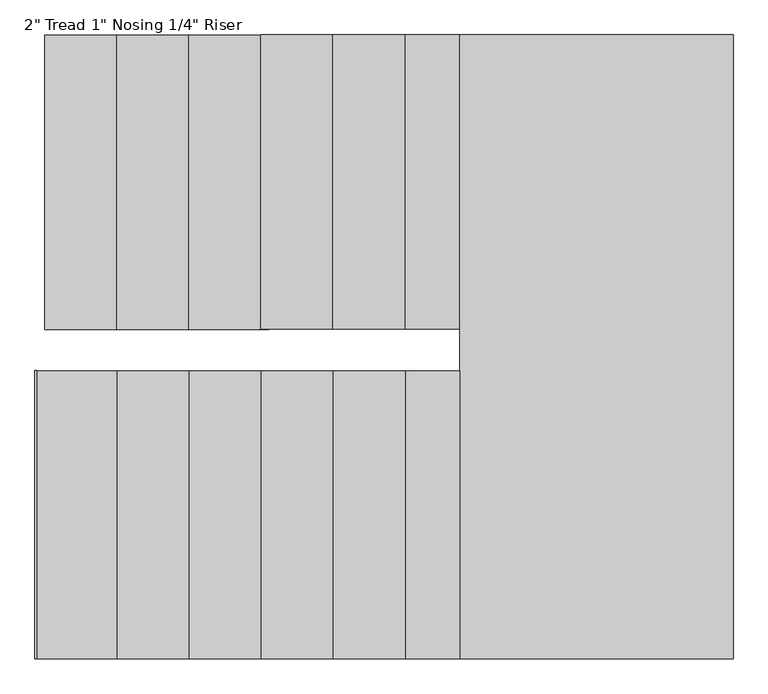
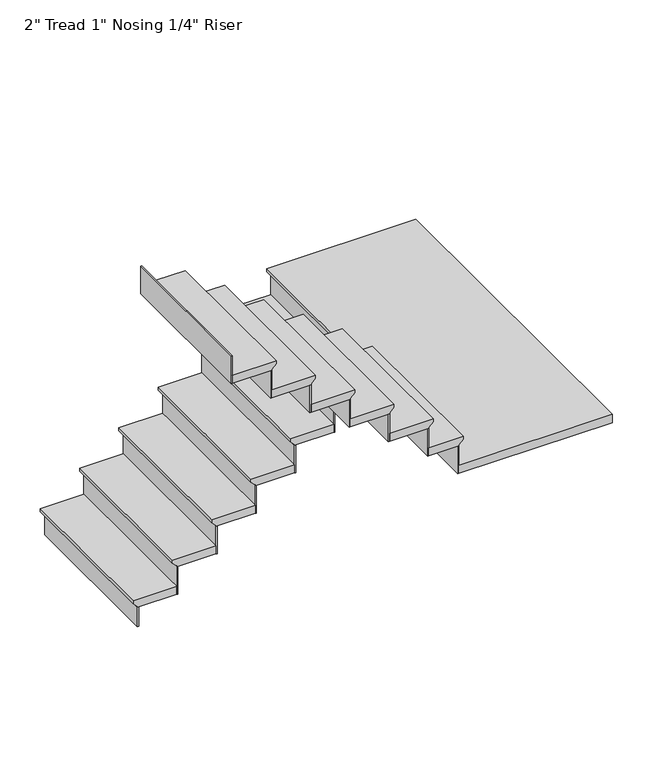
"""IFC4 building model written with IfcOpenShell, lengths in millimetres: stair flight geometry."""

from ifc_helpers import new_model, si_unit, origin, place, context, project, spatial, faceted_brep, source, transform, mapped, element, save


def stair_flight_9844eda0(model_context):
    return source(origin(), model_context, "Body", "Brep", [
        faceted_brep([(-1022.6415352, -3861.2539367, 3350.6833333), (-1022.6415352, -3861.2539367, 3369.7333333), (-1022.6415352, -2926.4769687, 3369.7333333), (-1022.6415352, -2926.4769687, 3350.6833333), (-997.2415352, -3861.2539367, 3325.2833333), (-997.2415352, -2926.4769687, 3325.2833333), (-768.6415352, -3861.2539367, 3369.7333333), (-768.6415352, -2926.4769687, 3369.7333333), (-997.2415352, -2926.4769687, 3318.9333333), (-768.6415352, -2926.4769687, 3318.9333333), (-768.6415352, -3861.2539367, 3318.9333333), (-997.2415352, -3861.2539367, 3318.9333333)], [[[0, 1, 2, 3]], [[4, 0, 3, 5]], [[2, 1, 6, 7]], [[8, 9, 10, 11]], [[2, 7, 9, 8, 5, 3]], [[8, 11, 4, 5]], [[6, 1, 0, 4, 11, 10]], [[7, 6, 10, 9]]]),
        faceted_brep([(-997.2415352, -3861.2539367, 3318.9333333), (-997.2415352, -3861.2539367, 3200.4), (-990.8915352, -3861.2539367, 3200.4), (-990.8915352, -3861.2539367, 3318.9333333), (-997.2415352, -2926.4769687, 3318.9333333), (-990.8915352, -2926.4769687, 3318.9333333), (-990.8915352, -2926.4769687, 3200.4), (-997.2415352, -2926.4769687, 3200.4)], [[[0, 1, 2, 3]], [[4, 5, 6, 7]], [[1, 0, 4, 7]], [[2, 1, 7, 6]], [[3, 2, 6, 5]], [[0, 3, 5, 4]]]),
        faceted_brep([(-768.6415352, -3861.2539367, 3488.2666667), (-768.6415352, -3861.2539367, 3318.9333333), (-762.2915352, -3861.2539367, 3318.9333333), (-762.2915352, -3861.2539367, 3488.2666667), (-768.6415352, -2926.4769687, 3488.2666667), (-762.2915352, -2926.4769687, 3488.2666667), (-762.2915352, -2926.4769687, 3318.9333333), (-768.6415352, -2926.4769687, 3318.9333333)], [[[0, 1, 2, 3]], [[4, 5, 6, 7]], [[1, 0, 4, 7]], [[2, 1, 7, 6]], [[3, 2, 6, 5]], [[0, 3, 5, 4]]]),
        faceted_brep([(-794.0415352, -2926.4769687, 3539.0666667), (-794.0415352, -3861.2539367, 3539.0666667), (-540.0415352, -3861.2539367, 3539.0666667), (-540.0415352, -2926.4769687, 3539.0666667), (-768.6415352, -2926.4769687, 3488.2666667), (-540.0415352, -2926.4769687, 3488.2666667), (-540.0415352, -3861.2539367, 3488.2666667), (-768.6415352, -3861.2539367, 3488.2666667), (-768.6415352, -2926.4769687, 3494.6166667), (-794.0415352, -2926.4769687, 3520.0166667), (-768.6415352, -3861.2539367, 3494.6166667), (-794.0415352, -3861.2539367, 3520.0166667)], [[[0, 1, 2, 3]], [[4, 5, 6, 7]], [[0, 3, 5, 4, 8, 9]], [[4, 7, 10, 8]], [[2, 1, 11, 10, 7, 6]], [[3, 2, 6, 5]], [[11, 1, 0, 9]], [[10, 11, 9, 8]]]),
        faceted_brep([(-540.0415352, -3861.2539367, 3657.6), (-540.0415352, -3861.2539367, 3488.2666667), (-533.6915352, -3861.2539367, 3488.2666667), (-533.6915352, -3861.2539367, 3657.6), (-540.0415352, -2926.4769687, 3657.6), (-533.6915352, -2926.4769687, 3657.6), (-533.6915352, -2926.4769687, 3488.2666667), (-540.0415352, -2926.4769687, 3488.2666667)], [[[0, 1, 2, 3]], [[4, 5, 6, 7]], [[1, 0, 4, 7]], [[2, 1, 7, 6]], [[3, 2, 6, 5]], [[0, 3, 5, 4]]]),
        faceted_brep([(-565.4415352, -2926.4769687, 3708.4), (-565.4415352, -3861.2539367, 3708.4), (-311.4415352, -3861.2539367, 3708.4), (-311.4415352, -2926.4769687, 3708.4), (-540.0415352, -2926.4769687, 3657.6), (-311.4415352, -2926.4769687, 3657.6), (-311.4415352, -3861.2539367, 3657.6), (-540.0415352, -3861.2539367, 3657.6), (-540.0415352, -2926.4769687, 3663.95), (-565.4415352, -2926.4769687, 3689.35), (-540.0415352, -3861.2539367, 3663.95), (-565.4415352, -3861.2539367, 3689.35)], [[[0, 1, 2, 3]], [[4, 5, 6, 7]], [[0, 3, 5, 4, 8, 9]], [[4, 7, 10, 8]], [[2, 1, 11, 10, 7, 6]], [[3, 2, 6, 5]], [[11, 1, 0, 9]], [[10, 11, 9, 8]]]),
        faceted_brep([(-311.4415352, -3861.2539367, 3826.9333333), (-311.4415352, -3861.2539367, 3657.6), (-305.0915352, -3861.2539367, 3657.6), (-305.0915352, -3861.2539367, 3826.9333333), (-311.4415352, -2926.4769687, 3826.9333333), (-305.0915352, -2926.4769687, 3826.9333333), (-305.0915352, -2926.4769687, 3657.6), (-311.4415352, -2926.4769687, 3657.6)], [[[0, 1, 2, 3]], [[4, 5, 6, 7]], [[1, 0, 4, 7]], [[2, 1, 7, 6]], [[3, 2, 6, 5]], [[0, 3, 5, 4]]]),
        faceted_brep([(-336.8415352, -2926.4769687, 3877.7333333), (-336.8415352, -3861.2539367, 3877.7333333), (-82.8415352, -3861.2539367, 3877.7333333), (-82.8415352, -2926.4769687, 3877.7333333), (-311.4415352, -2926.4769687, 3826.9333333), (-82.8415352, -2926.4769687, 3826.9333333), (-82.8415352, -3861.2539367, 3826.9333333), (-311.4415352, -3861.2539367, 3826.9333333), (-311.4415352, -2926.4769687, 3833.2833333), (-336.8415352, -2926.4769687, 3858.6833333), (-311.4415352, -3861.2539367, 3833.2833333), (-336.8415352, -3861.2539367, 3858.6833333)], [[[0, 1, 2, 3]], [[4, 5, 6, 7]], [[0, 3, 5, 4, 8, 9]], [[4, 7, 10, 8]], [[2, 1, 11, 10, 7, 6]], [[3, 2, 6, 5]], [[11, 1, 0, 9]], [[10, 11, 9, 8]]]),
        faceted_brep([(-82.8415352, -3861.2539367, 3996.2666667), (-82.8415352, -3861.2539367, 3826.9333333), (-76.4915352, -3861.2539367, 3826.9333333), (-76.4915352, -3861.2539367, 3996.2666667), (-82.8415352, -2926.4769687, 3996.2666667), (-76.4915352, -2926.4769687, 3996.2666667), (-76.4915352, -2926.4769687, 3826.9333333), (-82.8415352, -2926.4769687, 3826.9333333)], [[[0, 1, 2, 3]], [[4, 5, 6, 7]], [[1, 0, 4, 7]], [[2, 1, 7, 6]], [[3, 2, 6, 5]], [[0, 3, 5, 4]]]),
        faceted_brep([(-108.2415352, -2926.4769687, 4047.0666667), (-108.2415352, -3861.2539367, 4047.0666667), (145.7584648, -3861.2539367, 4047.0666667), (145.7584648, -2926.4769687, 4047.0666667), (-82.8415352, -2926.4769687, 3996.2666667), (145.7584648, -2926.4769687, 3996.2666667), (145.7584648, -3861.2539367, 3996.2666667), (-82.8415352, -3861.2539367, 3996.2666667), (-82.8415352, -2926.4769687, 4002.6166667), (-108.2415352, -2926.4769687, 4028.0166667), (-82.8415352, -3861.2539367, 4002.6166667), (-108.2415352, -3861.2539367, 4028.0166667)], [[[0, 1, 2, 3]], [[4, 5, 6, 7]], [[0, 3, 5, 4, 8, 9]], [[4, 7, 10, 8]], [[2, 1, 11, 10, 7, 6]], [[3, 2, 6, 5]], [[11, 1, 0, 9]], [[10, 11, 9, 8]]]),
        faceted_brep([(145.7584648, -3861.2539367, 4165.6), (145.7584648, -3861.2539367, 3996.2666667), (152.1084648, -3861.2539367, 3996.2666667), (152.1084648, -3861.2539367, 4165.6), (145.7584648, -2926.4769687, 4165.6), (152.1084648, -2926.4769687, 4165.6), (152.1084648, -2926.4769687, 3996.2666667), (145.7584648, -2926.4769687, 3996.2666667)], [[[0, 1, 2, 3]], [[4, 5, 6, 7]], [[1, 0, 4, 7]], [[2, 1, 7, 6]], [[3, 2, 6, 5]], [[0, 3, 5, 4]]]),
        faceted_brep([(120.3584648, -2926.4769687, 4216.4), (120.3584648, -3861.2539367, 4216.4), (320.0221038, -3861.2539367, 4216.4), (320.0221038, -2926.4769687, 4216.4), (145.7584648, -2926.4769687, 4165.6), (320.0221038, -2926.4769687, 4165.6), (320.0221038, -3861.2539367, 4165.6), (145.7584648, -3861.2539367, 4165.6), (145.7584648, -2926.4769687, 4171.95), (120.3584648, -2926.4769687, 4197.35), (145.7584648, -3861.2539367, 4171.95), (120.3584648, -3861.2539367, 4197.35)], [[[0, 1, 2, 3]], [[4, 5, 6, 7]], [[0, 3, 5, 4, 8, 9]], [[4, 7, 10, 8]], [[2, 1, 11, 10, 7, 6]], [[3, 2, 6, 5]], [[11, 1, 0, 9]], [[10, 11, 9, 8]]]),
        faceted_brep([(320.0221038, -3861.2539367, 4334.9333333), (320.0221038, -3861.2539367, 4165.6), (326.3721038, -3861.2539367, 4165.6), (326.3721038, -3861.2539367, 4334.9333333), (320.0221038, -2926.4769687, 4334.9333333), (326.3721038, -2926.4769687, 4334.9333333), (326.3721038, -2926.4769687, 4165.6), (320.0221038, -2926.4769687, 4165.6)], [[[0, 1, 2, 3]], [[4, 5, 6, 7]], [[1, 0, 4, 7]], [[2, 1, 7, 6]], [[3, 2, 6, 5]], [[0, 3, 5, 4]]]),
        faceted_brep([(269.2221038, -4907.6769687, 4385.7333333), (1161.7584648, -4907.6769687, 4385.7333333), (1161.7584648, -2926.4769687, 4385.7333333), (294.6221038, -2926.4769687, 4385.7333333), (294.6221038, -3993.2769687, 4385.7333333), (269.2221038, -3993.2769687, 4385.7333333), (1161.7584648, -4907.6769687, 4334.9333333), (269.2221038, -4907.6769687, 4334.9333333), (269.2221038, -3993.2769687, 4334.9333333), (294.6221038, -3993.2769687, 4334.9333333), (294.6221038, -3861.2539367, 4334.9333333), (320.0221038, -3861.2539367, 4334.9333333), (320.0221038, -2926.4769687, 4334.9333333), (1161.7584648, -2926.4769687, 4334.9333333), (320.0221038, -2926.4769687, 4341.2833333), (294.6221038, -2926.4769687, 4366.6833333), (320.0221038, -3861.2539367, 4341.2833333), (294.6221038, -3861.2539367, 4366.6833333)], [[[0, 1, 2, 3, 4, 5]], [[6, 7, 8, 9, 10, 11, 12, 13]], [[1, 0, 7, 6]], [[2, 1, 6, 13]], [[3, 2, 13, 12, 14, 15]], [[12, 11, 16, 14]], [[11, 10, 17, 16]], [[4, 3, 15, 17, 10, 9]], [[5, 4, 9, 8]], [[0, 5, 8, 7]], [[15, 14, 16, 17]]]),
        faceted_brep([(269.2221038, -3993.2769687, 4504.2666667), (269.2221038, -3993.2769687, 4334.9333333), (262.8721038, -3993.2769687, 4334.9333333), (262.8721038, -3993.2769687, 4504.2666667), (269.2221038, -4907.6769687, 4504.2666667), (262.8721038, -4907.6769687, 4504.2666667), (262.8721038, -4907.6769687, 4334.9333333), (269.2221038, -4907.6769687, 4334.9333333)], [[[0, 1, 2, 3]], [[4, 5, 6, 7]], [[1, 0, 4, 7]], [[2, 1, 7, 6]], [[3, 2, 6, 5]], [[0, 3, 5, 4]]]),
        faceted_brep([(294.6221038, -4907.6769687, 4555.0666667), (294.6221038, -3993.2769687, 4555.0666667), (94.9584648, -3993.2769687, 4555.0666667), (94.9584648, -4907.6769687, 4555.0666667), (269.2221038, -4907.6769687, 4504.2666667), (94.9584648, -4907.6769687, 4504.2666667), (94.9584648, -3993.2769687, 4504.2666667), (269.2221038, -3993.2769687, 4504.2666667), (269.2221038, -4907.6769687, 4510.6166667), (294.6221038, -4907.6769687, 4536.0166667), (269.2221038, -3993.2769687, 4510.6166667), (294.6221038, -3993.2769687, 4536.0166667)], [[[0, 1, 2, 3]], [[4, 5, 6, 7]], [[0, 3, 5, 4, 8, 9]], [[4, 7, 10, 8]], [[2, 1, 11, 10, 7, 6]], [[3, 2, 6, 5]], [[11, 1, 0, 9]], [[10, 11, 9, 8]]]),
        faceted_brep([(94.9584648, -3993.2769687, 4673.6), (94.9584648, -3993.2769687, 4504.2666667), (88.6084648, -3993.2769687, 4504.2666667), (88.6084648, -3993.2769687, 4673.6), (94.9584648, -4907.6769687, 4673.6), (88.6084648, -4907.6769687, 4673.6), (88.6084648, -4907.6769687, 4504.2666667), (94.9584648, -4907.6769687, 4504.2666667)], [[[0, 1, 2, 3]], [[4, 5, 6, 7]], [[1, 0, 4, 7]], [[2, 1, 7, 6]], [[3, 2, 6, 5]], [[0, 3, 5, 4]]]),
        faceted_brep([(120.3584648, -4907.6769687, 4724.4), (120.3584648, -3993.2769687, 4724.4), (-133.6415352, -3993.2769687, 4724.4), (-133.6415352, -4907.6769687, 4724.4), (94.9584648, -4907.6769687, 4673.6), (-133.6415352, -4907.6769687, 4673.6), (-133.6415352, -3993.2769687, 4673.6), (94.9584648, -3993.2769687, 4673.6), (94.9584648, -4907.6769687, 4679.95), (120.3584648, -4907.6769687, 4705.35), (94.9584648, -3993.2769687, 4679.95), (120.3584648, -3993.2769687, 4705.35)], [[[0, 1, 2, 3]], [[4, 5, 6, 7]], [[0, 3, 5, 4, 8, 9]], [[4, 7, 10, 8]], [[2, 1, 11, 10, 7, 6]], [[3, 2, 6, 5]], [[11, 1, 0, 9]], [[10, 11, 9, 8]]]),
        faceted_brep([(-133.6415352, -3993.2769687, 4842.9333333), (-133.6415352, -3993.2769687, 4673.6), (-139.9915352, -3993.2769687, 4673.6), (-139.9915352, -3993.2769687, 4842.9333333), (-133.6415352, -4907.6769687, 4842.9333333), (-139.9915352, -4907.6769687, 4842.9333333), (-139.9915352, -4907.6769687, 4673.6), (-133.6415352, -4907.6769687, 4673.6)], [[[0, 1, 2, 3]], [[4, 5, 6, 7]], [[1, 0, 4, 7]], [[2, 1, 7, 6]], [[3, 2, 6, 5]], [[0, 3, 5, 4]]]),
        faceted_brep([(-108.2415352, -4907.6769687, 4893.7333333), (-108.2415352, -3993.2769687, 4893.7333333), (-362.2415352, -3993.2769687, 4893.7333333), (-362.2415352, -4907.6769687, 4893.7333333), (-133.6415352, -4907.6769687, 4842.9333333), (-362.2415352, -4907.6769687, 4842.9333333), (-362.2415352, -3993.2769687, 4842.9333333), (-133.6415352, -3993.2769687, 4842.9333333), (-133.6415352, -4907.6769687, 4849.2833333), (-108.2415352, -4907.6769687, 4874.6833333), (-133.6415352, -3993.2769687, 4849.2833333), (-108.2415352, -3993.2769687, 4874.6833333)], [[[0, 1, 2, 3]], [[4, 5, 6, 7]], [[0, 3, 5, 4, 8, 9]], [[4, 7, 10, 8]], [[2, 1, 11, 10, 7, 6]], [[3, 2, 6, 5]], [[11, 1, 0, 9]], [[10, 11, 9, 8]]]),
        faceted_brep([(-362.2415352, -3993.2769687, 5012.2666667), (-362.2415352, -3993.2769687, 4842.9333333), (-368.5915352, -3993.2769687, 4842.9333333), (-368.5915352, -3993.2769687, 5012.2666667), (-362.2415352, -4907.6769687, 5012.2666667), (-368.5915352, -4907.6769687, 5012.2666667), (-368.5915352, -4907.6769687, 4842.9333333), (-362.2415352, -4907.6769687, 4842.9333333)], [[[0, 1, 2, 3]], [[4, 5, 6, 7]], [[1, 0, 4, 7]], [[2, 1, 7, 6]], [[3, 2, 6, 5]], [[0, 3, 5, 4]]]),
        faceted_brep([(-336.8415352, -4907.6769687, 5063.0666667), (-336.8415352, -3993.2769687, 5063.0666667), (-590.8415352, -3993.2769687, 5063.0666667), (-590.8415352, -4907.6769687, 5063.0666667), (-362.2415352, -4907.6769687, 5012.2666667), (-590.8415352, -4907.6769687, 5012.2666667), (-590.8415352, -3993.2769687, 5012.2666667), (-362.2415352, -3993.2769687, 5012.2666667), (-362.2415352, -4907.6769687, 5018.6166667), (-336.8415352, -4907.6769687, 5044.0166667), (-362.2415352, -3993.2769687, 5018.6166667), (-336.8415352, -3993.2769687, 5044.0166667)], [[[0, 1, 2, 3]], [[4, 5, 6, 7]], [[0, 3, 5, 4, 8, 9]], [[4, 7, 10, 8]], [[2, 1, 11, 10, 7, 6]], [[3, 2, 6, 5]], [[11, 1, 0, 9]], [[10, 11, 9, 8]]]),
        faceted_brep([(-590.8415352, -3993.2769687, 5181.6), (-590.8415352, -3993.2769687, 5012.2666667), (-597.1915352, -3993.2769687, 5012.2666667), (-597.1915352, -3993.2769687, 5181.6), (-590.8415352, -4907.6769687, 5181.6), (-597.1915352, -4907.6769687, 5181.6), (-597.1915352, -4907.6769687, 5012.2666667), (-590.8415352, -4907.6769687, 5012.2666667)], [[[0, 1, 2, 3]], [[4, 5, 6, 7]], [[1, 0, 4, 7]], [[2, 1, 7, 6]], [[3, 2, 6, 5]], [[0, 3, 5, 4]]]),
        faceted_brep([(-565.4415352, -4907.6769687, 5232.4), (-565.4415352, -3993.2769687, 5232.4), (-819.4415352, -3993.2769687, 5232.4), (-819.4415352, -4907.6769687, 5232.4), (-590.8415352, -4907.6769687, 5181.6), (-819.4415352, -4907.6769687, 5181.6), (-819.4415352, -3993.2769687, 5181.6), (-590.8415352, -3993.2769687, 5181.6), (-590.8415352, -4907.6769687, 5187.95), (-565.4415352, -4907.6769687, 5213.35), (-590.8415352, -3993.2769687, 5187.95), (-565.4415352, -3993.2769687, 5213.35)], [[[0, 1, 2, 3]], [[4, 5, 6, 7]], [[0, 3, 5, 4, 8, 9]], [[4, 7, 10, 8]], [[2, 1, 11, 10, 7, 6]], [[3, 2, 6, 5]], [[11, 1, 0, 9]], [[10, 11, 9, 8]]]),
        faceted_brep([(-819.4415352, -3993.2769687, 5350.9333333), (-819.4415352, -3993.2769687, 5181.6), (-825.7915352, -3993.2769687, 5181.6), (-825.7915352, -3993.2769687, 5350.9333333), (-819.4415352, -4907.6769687, 5350.9333333), (-825.7915352, -4907.6769687, 5350.9333333), (-825.7915352, -4907.6769687, 5181.6), (-819.4415352, -4907.6769687, 5181.6)], [[[0, 1, 2, 3]], [[4, 5, 6, 7]], [[1, 0, 4, 7]], [[2, 1, 7, 6]], [[3, 2, 6, 5]], [[0, 3, 5, 4]]]),
        faceted_brep([(-1048.0415352, -3993.2769687, 5520.2666667), (-1048.0415352, -3993.2769687, 5350.9333333), (-1054.3915352, -3993.2769687, 5350.9333333), (-1054.3915352, -3993.2769687, 5520.2666667), (-1048.0415352, -4907.6769687, 5520.2666667), (-1054.3915352, -4907.6769687, 5520.2666667), (-1054.3915352, -4907.6769687, 5350.9333333), (-1048.0415352, -4907.6769687, 5350.9333333)], [[[0, 1, 2, 3]], [[4, 5, 6, 7]], [[1, 0, 4, 7]], [[2, 1, 7, 6]], [[3, 2, 6, 5]], [[0, 3, 5, 4]]]),
        faceted_brep([(-794.0415352, -4907.6769687, 5401.7333333), (-794.0415352, -3993.2769687, 5401.7333333), (-1048.0415352, -3993.2769687, 5401.7333333), (-1048.0415352, -4907.6769687, 5401.7333333), (-819.4415352, -4907.6769687, 5350.9333333), (-1048.0415352, -4907.6769687, 5350.9333333), (-1048.0415352, -3993.2769687, 5350.9333333), (-819.4415352, -3993.2769687, 5350.9333333), (-819.4415352, -4907.6769687, 5357.2833333), (-794.0415352, -4907.6769687, 5382.6833333), (-819.4415352, -3993.2769687, 5357.2833333), (-794.0415352, -3993.2769687, 5382.6833333)], [[[0, 1, 2, 3]], [[4, 5, 6, 7]], [[0, 3, 5, 4, 8, 9]], [[4, 7, 10, 8]], [[2, 1, 11, 10, 7, 6]], [[3, 2, 6, 5]], [[11, 1, 0, 9]], [[10, 11, 9, 8]]]),
    ])


if __name__ == "__main__":
    model = new_model("IFC4")
    model_context = context("Model", 3, world=origin())
    ifc_project = project(units=[si_unit("LENGTHUNIT", "METRE", prefix="MILLI")], contexts=[model_context])
    site = spatial("IfcSite", under=ifc_project)
    building = spatial("IfcBuilding", under=site)
    placement = place(None, origin())
    stair_flight_shape = stair_flight_9844eda0(model_context)
    element("IfcStairFlight", 1, ObjectType="2\" Tread 1\" Nosing 1/4\" Riser", at=placement, inside=building, context=model_context, shape_type="MappedRepresentation", body=[
        mapped(stair_flight_shape, transform((0.0, 0.0, 0.0), x_axis=(1.0, 0.0, 0.0), y_axis=(0.0, 1.0, 0.0), z_axis=(0.0, 0.0, 1.0))),
    ])
    save(model, "model.ifc")
